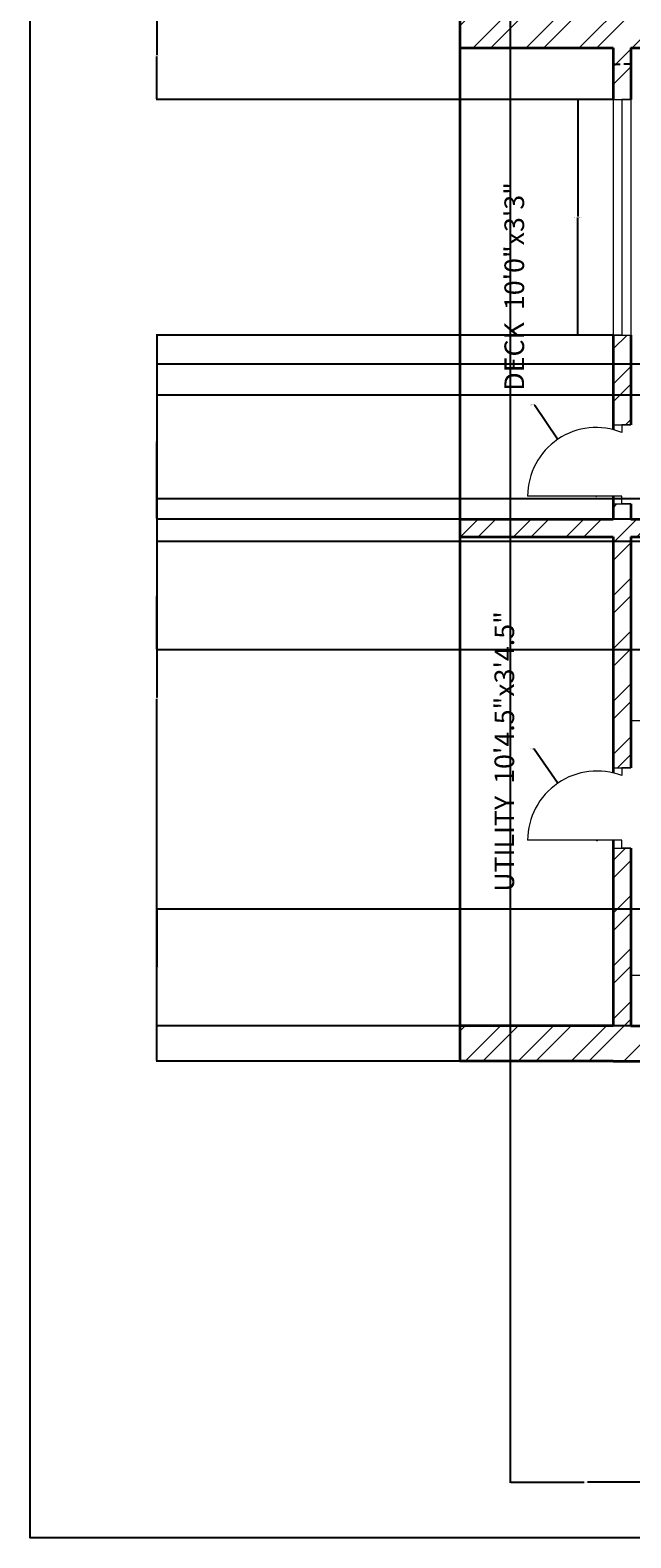
# Model space of a CAD drawing. Units: inches. Extents: x 1748 to 2382, y 1346 to 2284.
# Tile 1 of 26: x 1748 to 1901, y 1346 to 1730. Entities that reach past the tile are written whole.
import ezdxf

# ---------------------------------------------------------------- set-up
doc = ezdxf.new("R2010")
doc.units = ezdxf.units.IN
for name, color, linetype, lineweight in [('A-ANNO-DIMS', 2, 'Continuous', 18), ('A-ANNO-TTLB', 7, 'Continuous', 25), ('A-AREA-IDEN', 7, 'Continuous', 18), ('A-DOOR', 21, 'Continuous', 18), ('A-FLOR-CASE', 32, 'Continuous', 18), ('A-GLAZ', 191, 'Continuous', 18), ('A-WALL', 7, 'Continuous', 35), ('A-WALL-PATT', 9, 'Continuous', 13)]:
    doc.layers.add(name, color=color, linetype=linetype, lineweight=lineweight)
doc.styles.get("Standard").update_dxf_attribs({"font": 'arial.ttf'})
doc.dimstyles.get("Standard").update_dxf_attribs({"dimtxt": 0.18, "dimasz": 0.18, "dimexe": 0.18, "dimexo": 0.0625, "dimgap": 0.09, "dimtad": 0, "dimtih": 1, "dimtoh": 1, "dimdec": 4, "dimzin": 0, "dimdsep": 46, "dimtxsty": 'Standard', "dimcen": 0.09, "dimadec": 0, "dimazin": 0, "dimtfac": 1, "dimtdec": 4, "dimtofl": 0, "dimtmove": 0, "dimatfit": 3, "dimfxl": 1, "dimtolj": 1, "dimtzin": 0, "dimarcsym": 0})

# ---------------------------------------------------------------- blocks, each defined once
blk = doc.blocks.new('WIN-60-SHALLOW')
for p, q in [((0, 60), (4.5, 60)), ((0, 60), (0, 0)), ((4.5, 60), (2.25, 60)), ((2.25, 60), (2.25, 0)), ((4.5, 60), (4.5, 0)), ((2.25, 0), (0, 0)), ((0, 0), (4.5, 0))]:
    blk.add_line(p, q)
blk = doc.blocks.new('*D30')
at = {"layer": 'A-ANNO-DIMS', "color": 0, "lineweight": -2, "transparency": 16777216}
for p, q in [((1896.08, 1712.72), (1886.96, 1712.72)), ((1887.14, 1712.54), (1887.14, 1682.91)), ((1887.14, 1652.9), (1887.14, 1682.54)), ((1896.08, 1652.72), (1886.96, 1652.72))]:
    blk.add_line(p, q, dxfattribs=at)
at = {"layer": 'A-ANNO-DIMS', "color": 0, "transparency": 16777216}
for points in [[(1887.11, 1712.54), (1887.17, 1712.54), (1887.14, 1712.72)], [(1887.11, 1652.9), (1887.17, 1652.9), (1887.14, 1652.72)]]:
    blk.add_solid(points, dxfattribs=at)
at = {"layer": 'Defpoints', "color": 0, "transparency": 16777216}
for p in [(1887.14, 1712.72), (1896.14, 1712.72), (1896.14, 1652.72)]:
    blk.add_point(p, dxfattribs=at)
at = {"layer": 'A-ANNO-DIMS', "color": 0, "transparency": 16777216, "insert": (1887.14, 1682.72), "char_height": 0.18, "attachment_point": 5}
blk.add_mtext('\\A1;WINDOW 60 TYP.', dxfattribs=at)
blk = doc.blocks.new('*D31')
at = {"layer": 'A-ANNO-DIMS', "color": 0, "lineweight": -2, "transparency": 16777216}
for p, q in [((1896.14, 1712.79), (1896.14, 1721.9)), ((1896.32, 1721.72), (1897.93, 1721.72)), ((1900.46, 1721.72), (1898.85, 1721.72)), ((1900.64, 1712.79), (1900.64, 1721.9))]:
    blk.add_line(p, q, dxfattribs=at)
at = {"layer": 'A-ANNO-DIMS', "color": 0, "transparency": 16777216}
for points in [[(1896.32, 1721.75), (1896.32, 1721.69), (1896.14, 1721.72)], [(1900.46, 1721.75), (1900.46, 1721.69), (1900.64, 1721.72)]]:
    blk.add_solid(points, dxfattribs=at)
at = {"layer": 'Defpoints', "color": 0, "transparency": 16777216}
for p in [(1900.64, 1721.72), (1896.14, 1712.72), (1900.64, 1712.72)]:
    blk.add_point(p, dxfattribs=at)
at = {"layer": 'A-ANNO-DIMS', "color": 0, "transparency": 16777216, "insert": (1898.39, 1721.72), "char_height": 0.18, "attachment_point": 5}
blk.add_mtext('\\A1;5 TYP.', dxfattribs=at)
blk = doc.blocks.new('*D42')
at = {"layer": 'A-ANNO-DIMS', "color": 0, "lineweight": -2, "transparency": 16777216}
for p, q in [((1896.08, 1652.72), (1779.88, 1652.72)), ((1780.06, 1652.54), (1780.06, 1560.47)), ((1780.06, 1468.03), (1780.06, 1560.1)), ((1857.08, 1467.85), (1779.88, 1467.85))]:
    blk.add_line(p, q, dxfattribs=at)
at = {"layer": 'A-ANNO-DIMS', "color": 0, "transparency": 16777216}
for points in [[(1780.03, 1652.54), (1780.09, 1652.54), (1780.06, 1652.72)], [(1780.03, 1468.03), (1780.09, 1468.03), (1780.06, 1467.85)]]:
    blk.add_solid(points, dxfattribs=at)
at = {"layer": 'Defpoints', "color": 0, "transparency": 16777216}
for p in [(1780.06, 1652.72), (1896.14, 1652.72), (1857.14, 1467.85)]:
    blk.add_point(p, dxfattribs=at)
at = {"layer": 'A-ANNO-DIMS', "color": 0, "transparency": 16777216, "insert": (1780.06, 1560.29), "char_height": 0.18, "attachment_point": 5}
blk.add_mtext('\\A1;184.87', dxfattribs=at)
blk = doc.blocks.new('*D50')
at = {"layer": 'A-ANNO-DIMS', "color": 0, "lineweight": -2, "transparency": 16777216}
for p, q in [((1869.96, 2223.79), (1869.96, 1360.47)), ((1908.44, 2223.79), (1908.44, 1360.47)), ((1870.14, 1360.65), (1888.81, 1360.65)), ((1908.26, 1360.65), (1889.6, 1360.65))]:
    blk.add_line(p, q, dxfattribs=at)
at = {"layer": 'A-ANNO-DIMS', "color": 0, "transparency": 16777216}
for points in [[(1870.14, 1360.68), (1870.14, 1360.62), (1869.96, 1360.65)], [(1908.26, 1360.68), (1908.26, 1360.62), (1908.44, 1360.65)]]:
    blk.add_solid(points, dxfattribs=at)
at = {"layer": 'Defpoints', "color": 0, "transparency": 16777216}
for p in [(1869.96, 2223.85), (1908.44, 2223.85), (1908.44, 1360.65)]:
    blk.add_point(p, dxfattribs=at)
at = {"layer": 'A-ANNO-DIMS', "color": 0, "transparency": 16777216, "insert": (1889.2, 1360.65), "char_height": 0.18, "attachment_point": 5}
blk.add_mtext('\\A1;38.48', dxfattribs=at)
blk = doc.blocks.new('*D54')
at = {"layer": 'A-ANNO-DIMS', "color": 0, "lineweight": -2, "transparency": 16777216}
for p, q in [((2288.4, 1506.57), (1779.88, 1506.57)), ((1780.06, 1506.39), (1780.06, 1491.89)), ((1780.06, 1477.03), (1780.06, 1491.53)), ((2288.4, 1476.85), (1779.88, 1476.85))]:
    blk.add_line(p, q, dxfattribs=at)
at = {"layer": 'A-ANNO-DIMS', "color": 0, "transparency": 16777216}
for points in [[(1780.03, 1506.39), (1780.09, 1506.39), (1780.06, 1506.57)], [(1780.03, 1477.03), (1780.09, 1477.03), (1780.06, 1476.85)]]:
    blk.add_solid(points, dxfattribs=at)
at = {"layer": 'Defpoints', "color": 0, "transparency": 16777216}
for p in [(1780.06, 1506.57), (2288.46, 1506.57), (2288.46, 1476.85)]:
    blk.add_point(p, dxfattribs=at)
at = {"layer": 'A-ANNO-DIMS', "color": 0, "transparency": 16777216, "insert": (1780.06, 1491.71), "char_height": 0.18, "attachment_point": 5}
blk.add_mtext('\\A1;29.716', dxfattribs=at)
blk = doc.blocks.new('*D55')
at = {"layer": 'A-ANNO-DIMS', "color": 0, "lineweight": -2, "transparency": 16777216}
for p, q in [((2288.4, 1645.3), (1779.88, 1645.3)), ((1780.06, 1645.12), (1780.06, 1625.76)), ((1780.06, 1606.03), (1780.06, 1625.39)), ((2288.4, 1605.85), (1779.88, 1605.85))]:
    blk.add_line(p, q, dxfattribs=at)
at = {"layer": 'A-ANNO-DIMS', "color": 0, "transparency": 16777216}
for points in [[(1780.03, 1645.12), (1780.09, 1645.12), (1780.06, 1645.3)], [(1780.03, 1606.03), (1780.09, 1606.03), (1780.06, 1605.85)]]:
    blk.add_solid(points, dxfattribs=at)
at = {"layer": 'Defpoints', "color": 0, "transparency": 16777216}
for p in [(1780.06, 1645.3), (2288.46, 1645.3), (2288.46, 1605.85)]:
    blk.add_point(p, dxfattribs=at)
at = {"layer": 'A-ANNO-DIMS', "color": 0, "transparency": 16777216, "insert": (1780.06, 1625.58), "char_height": 0.18, "attachment_point": 5}
blk.add_mtext('\\A1;39.454', dxfattribs=at)
blk = doc.blocks.new('*D71')
at = {"layer": 'A-ANNO-DIMS', "color": 0, "lineweight": -2, "transparency": 16777216}
for p, q in [((1857.08, 1734.85), (1779.88, 1734.85)), ((1780.06, 1734.67), (1780.06, 1723.97)), ((1780.06, 1712.9), (1780.06, 1723.61)), ((1896.08, 1712.72), (1779.88, 1712.72))]:
    blk.add_line(p, q, dxfattribs=at)
at = {"layer": 'A-ANNO-DIMS', "color": 0, "transparency": 16777216}
for points in [[(1780.03, 1734.67), (1780.09, 1734.67), (1780.06, 1734.85)], [(1780.03, 1712.9), (1780.09, 1712.9), (1780.06, 1712.72)]]:
    blk.add_solid(points, dxfattribs=at)
at = {"layer": 'Defpoints', "color": 0, "transparency": 16777216}
for p in [(1780.06, 1734.85), (1857.14, 1734.85), (1896.14, 1712.72)]:
    blk.add_point(p, dxfattribs=at)
at = {"layer": 'A-ANNO-DIMS', "color": 0, "transparency": 16777216, "insert": (1780.06, 1723.79), "char_height": 0.18, "attachment_point": 5}
blk.add_mtext('\\A1;22.127', dxfattribs=at)
blk = doc.blocks.new('*D74')
at = {"layer": 'A-ANNO-DIMS', "color": 0, "lineweight": -2, "transparency": 16777216}
for p, q in [((2006.4, 1637.45), (1779.88, 1637.45)), ((1780.06, 1637.27), (1780.06, 1624.43)), ((1780.06, 1611.24), (1780.06, 1624.07)), ((2006.4, 1611.06), (1779.88, 1611.06))]:
    blk.add_line(p, q, dxfattribs=at)
at = {"layer": 'A-ANNO-DIMS', "color": 0, "transparency": 16777216}
for points in [[(1780.03, 1637.27), (1780.09, 1637.27), (1780.06, 1637.45)], [(1780.03, 1611.24), (1780.09, 1611.24), (1780.06, 1611.06)]]:
    blk.add_solid(points, dxfattribs=at)
at = {"layer": 'Defpoints', "color": 0, "transparency": 16777216}
for p in [(1780.06, 1637.45), (2006.46, 1637.45), (2006.46, 1611.06)]:
    blk.add_point(p, dxfattribs=at)
at = {"layer": 'A-ANNO-DIMS', "color": 0, "transparency": 16777216, "insert": (1780.06, 1624.25), "char_height": 0.18, "attachment_point": 5}
blk.add_mtext('\\A1;26.39', dxfattribs=at)
blk = doc.blocks.new('*D80')
at = {"layer": 'A-ANNO-DIMS', "color": 0, "lineweight": -2, "transparency": 16777216}
for p, q in [((2058.9, 1600.19), (1779.88, 1600.19)), ((1780.06, 1600.01), (1780.06, 1586.55)), ((1780.06, 1572.73), (1780.06, 1586.19)), ((2058.9, 1572.55), (1779.88, 1572.55))]:
    blk.add_line(p, q, dxfattribs=at)
at = {"layer": 'A-ANNO-DIMS', "color": 0, "transparency": 16777216}
for points in [[(1780.03, 1600.01), (1780.09, 1600.01), (1780.06, 1600.19)], [(1780.03, 1572.73), (1780.09, 1572.73), (1780.06, 1572.55)]]:
    blk.add_solid(points, dxfattribs=at)
at = {"layer": 'Defpoints', "color": 0, "transparency": 16777216}
for p in [(1780.06, 1600.19), (2058.96, 1600.19), (2058.96, 1572.55)]:
    blk.add_point(p, dxfattribs=at)
at = {"layer": 'A-ANNO-DIMS', "color": 0, "transparency": 16777216, "insert": (1780.06, 1586.37), "char_height": 0.18, "attachment_point": 5}
blk.add_mtext('\\A1;27.637', dxfattribs=at)
blk = doc.blocks.new('*D93')
at = {"layer": 'A-ANNO-DIMS', "color": 0, "lineweight": -2, "transparency": 16777216}
for p, q in [((1875.89, 1547.36), (1876.07, 1547.36)), ((1876.07, 1547.36), (1881.96, 1538.78)), ((1891.95, 1524.08), (1892.13, 1524.08)), ((1892.04, 1523.99), (1892.04, 1524.17))]:
    blk.add_line(p, q, dxfattribs=at)
at = {"layer": 'A-ANNO-DIMS', "color": 0, "transparency": 16777216}
blk.add_solid([(1881.98, 1538.8), (1881.93, 1538.77), (1882.06, 1538.63)], dxfattribs=at)
at = {"layer": 'Defpoints', "color": 0, "transparency": 16777216}
for p in [(1882.06, 1538.63), (1892.04, 1524.08)]:
    blk.add_point(p, dxfattribs=at)
at = {"layer": 'A-ANNO-DIMS', "color": 0, "transparency": 16777216, "insert": (1875.34, 1547.36), "char_height": 0.18, "attachment_point": 5}
blk.add_mtext('\\A1;R17.646', dxfattribs=at)
blk = doc.blocks.new('*D95')
at = {"layer": 'A-ANNO-DIMS', "color": 0, "lineweight": -2, "transparency": 16777216}
for p, q in [((1876.05, 1634.88), (1876.23, 1634.88)), ((1876.23, 1634.88), (1881.99, 1626.34)), ((1891.76, 1611.72), (1891.94, 1611.72)), ((1891.85, 1611.63), (1891.85, 1611.81))]:
    blk.add_line(p, q, dxfattribs=at)
at = {"layer": 'A-ANNO-DIMS', "color": 0, "transparency": 16777216}
blk.add_solid([(1882.01, 1626.36), (1881.96, 1626.32), (1882.09, 1626.19)], dxfattribs=at)
at = {"layer": 'Defpoints', "color": 0, "transparency": 16777216}
for p in [(1882.09, 1626.19), (1891.85, 1611.72)]:
    blk.add_point(p, dxfattribs=at)
at = {"layer": 'A-ANNO-DIMS', "color": 0, "transparency": 16777216, "insert": (1875.5, 1634.88), "char_height": 0.18, "attachment_point": 5}
blk.add_mtext('\\A1;R17.458', dxfattribs=at)

msp = doc.modelspace()

# ---------------------------------------------------------------- hatches: boundary and pattern name
at = {"layer": 'A-WALL-PATT'}
h = msp.add_hatch(dxfattribs=at)
h.set_pattern_fill('ANSI32', color=256)
h.paths.add_polyline_path([(1908.4445, 2232.8497), (1821.9607, 2232.8497), (1821.9607, 2223.8497), (1865.4607, 2223.8497), (1865.4607, 2209.9185), (1869.9607, 2209.9185), (1869.9607, 2223.8497), (1908.4445, 2223.8497), (1908.4445, 2228.3497)])
h.paths.add_polyline_path([(2040.0683, 2232.8497), (1968.4445, 2232.8497), (1968.4445, 2223.8497), (2025.9607, 2223.8497), (2025.9607, 2130.3497), (2032.1341, 2130.3497), (2032.1341, 2132.5997), (2032.1341, 2134.8497), (2030.4607, 2134.8497), (2030.4607, 2223.8497), (2040.0683, 2223.8497)])
h.paths.add_polyline_path([(2091.3969, 2232.8497), (2064.0683, 2232.8497), (2064.0683, 2223.8497), (2078.4607, 2223.8497), (2078.4607, 2134.8497), (2051.1563, 2134.8497), (2051.1563, 2130.3497), (2078.4607, 2130.3497), (2078.4607, 2128.6813), (2082.9607, 2128.6813), (2082.9607, 2130.3497), (2086.1879, 2130.3497), (2086.1879, 2132.5997), (2086.1879, 2134.8497), (2082.9607, 2134.8497), (2082.9607, 2223.8497), (2091.3969, 2223.8497), (2091.3969, 2228.3497)])
h.paths.add_polyline_path([(2167.0164, 2232.8497), (2115.3969, 2232.8497), (2115.3969, 2223.8497), (2130.9607, 2223.8497), (2130.9607, 2134.8497), (2106.9607, 2134.8497), (2106.9607, 2130.3497), (2135.4607, 2130.3497), (2135.4607, 2223.8497), (2167.0164, 2223.8497), (2167.0164, 2228.3497)])
h.paths.add_polyline_path([(1869.9607, 2149.9185), (1865.4607, 2149.9185), (1865.4607, 2127.8942), (1869.9607, 2127.8942)])
h.paths.add_polyline_path([(2082.9607, 2104.4871), (2080.7107, 2104.4871), (2078.4607, 2104.4871), (2078.4607, 2103.8497), (1869.9607, 2103.8497), (1869.9607, 2108.6062), (1867.7107, 2108.6062), (1865.4607, 2108.6062), (1865.4607, 2103.8497), (1821.9607, 2103.8497), (1821.9607, 2099.3497), (1865.4607, 2099.3497), (1865.4607, 2094.7509), (1869.9607, 2094.7509), (1869.9607, 2099.3497), (2025.9607, 2099.3497), (2025.9607, 2096.4326), (2030.4607, 2096.4326), (2030.4607, 2099.3497), (2082.9607, 2099.3497)])
h.paths.add_polyline_path([(1928.9457, 1401.1212), (2176.8693, 1401.1212), (2176.8693, 1438.214), (1928.9457, 1438.214)], flags=9)
h.paths.add_polyline_path([(2122.2668, 2048.1927), (2177.9387, 2048.1927), (2177.9387, 2066.85), (2122.2668, 2066.85)], flags=9)
h.paths.add_polyline_path([(2272.688, 2153.8197), (2272.688, 2216.746), (2262.3845, 2216.746), (2262.3845, 2153.8197)], flags=9)
h.paths.add_polyline_path([(2157.2928, 2166.5593), (2196.3822, 2166.5593), (2196.3822, 2185.2167), (2157.2928, 2185.2167)], flags=9)
h.paths.add_polyline_path([(2089.3407, 2162.0698), (2124.3987, 2162.0698), (2124.3987, 2180.7272), (2089.3407, 2180.7272)], flags=9)
h.paths.add_polyline_path([(2037.4521, 2160.0913), (2072.5101, 2160.0913), (2072.5101, 2178.7486), (2037.4521, 2178.7486)], flags=9)
h.paths.add_polyline_path([(1884.7894, 2104.1554), (1923.6297, 2104.1554), (1923.6297, 2122.8127), (1884.7894, 2122.8127)], flags=9)
h.paths.add_polyline_path([(1851.2832, 2142.9749), (1851.2832, 2199.3051), (1840.9796, 2199.3051), (1840.9796, 2142.9749)], flags=9)
h.paths.add_polyline_path([(1844.8763, 2017.2834), (1844.8763, 2073.6136), (1834.5728, 2073.6136), (1834.5728, 2017.2834)], flags=9)
h.paths.add_polyline_path([(1897.1577, 2073.1279), (1935.9981, 2073.1279), (1935.9981, 2091.7853), (1897.1577, 2091.7853)], flags=9)
h.paths.add_polyline_path([(1952.3395, 1802.4231), (2008.0114, 1802.4231), (2008.0114, 1821.0805), (1952.3395, 1821.0805)], flags=9)
h.paths.add_polyline_path([(1978.8184, 1857.6841), (2017.7338, 1857.6841), (2017.7338, 1876.3415), (1978.8184, 1876.3415)], flags=9)
h.paths.add_polyline_path([(1979.6513, 1925.9516), (2008.8089, 1925.9516), (2008.8089, 1944.6089), (1979.6513, 1944.6089)], flags=9)
h.paths.add_polyline_path([(1838.5553, 1860.3527), (1877.3957, 1860.3527), (1877.3957, 1879.01), (1838.5553, 1879.01)], flags=9)
h.paths.add_polyline_path([(1883.9018, 1787.3013), (1883.9018, 1843.6315), (1873.5983, 1843.6315), (1873.5983, 1787.3013)], flags=9)
h.paths.add_polyline_path([(1873.7079, 1509.1938), (1873.7079, 1583.7709), (1863.4044, 1583.7709), (1863.4044, 1509.1938)], flags=9)
h.paths.add_polyline_path([(1916.2259, 1603.3681), (1955.0663, 1603.3681), (1955.0663, 1622.0254), (1916.2259, 1622.0254)], flags=9)
h.paths.add_polyline_path([(1876.3013, 1636.757), (1876.3013, 1693.0871), (1865.9978, 1693.0871), (1865.9978, 1636.757)], flags=9)
h.paths.add_polyline_path([(1921.3138, 1521.8316), (1964.0662, 1521.8316), (1964.0662, 1540.489), (1921.3138, 1540.489)], flags=9)
h.paths.add_polyline_path([(2017.5657, 1497.5078), (2046.7983, 1497.5078), (2046.7983, 1516.1651), (2017.5657, 1516.1651)], flags=9)
h.paths.add_polyline_path([(2066.8661, 1499.3902), (2096.0988, 1499.3902), (2096.0988, 1518.0475), (2066.8661, 1518.0475)], flags=9)
h.paths.add_polyline_path([(2155.4835, 1571.6596), (2198.2358, 1571.6596), (2198.2358, 1590.3169), (2155.4835, 1590.3169)], flags=9)
h.paths.add_polyline_path([(2094.9136, 1664.6812), (2150.5855, 1664.6812), (2150.5855, 1683.3386), (2094.9136, 1683.3386)], flags=9)
h.paths.add_polyline_path([(2257.6902, 1863.1628), (2269.8935, 1863.1628), (2269.8935, 1873.4664), (2257.6902, 1873.4664)], flags=9)
h.paths.add_polyline_path([(2164.0748, 1880.3089), (2189.8694, 1880.3089), (2189.8694, 1890.6124), (2164.0748, 1890.6124)], flags=9)
h.paths.add_polyline_path([(2239.4394, 1931.0585), (2268.8187, 1931.0585), (2268.8187, 1949.7159), (2239.4394, 1949.7159)], flags=9)
h = msp.add_hatch(dxfattribs=at)
h.set_pattern_fill('ANSI32', color=256)
h.paths.add_polyline_path([(2297.4607, 2232.8497), (2203.0164, 2232.8497), (2203.0164, 2223.8497), (2244.9607, 2223.8497), (2244.9607, 2127.8554), (2249.4607, 2127.8554), (2249.4607, 2223.8497), (2297.4607, 2223.8497)])
h.paths.add_polyline_path([(2297.4607, 2103.8497), (2249.4607, 2103.8497), (2249.4607, 2106.7497), (2247.2107, 2106.7497), (2244.9607, 2106.7497), (2244.9607, 2103.8497), (2130.9607, 2103.8497), (2130.9607, 2099.3497), (2288.4607, 2099.3497), (2288.4607, 2077.2008), (2297.4607, 2077.2008)])
h.paths.add_polyline_path([(1928.9457, 1401.1212), (2176.8693, 1401.1212), (2176.8693, 1438.214), (1928.9457, 1438.214)], flags=9)
h.paths.add_polyline_path([(2122.2668, 2048.1927), (2177.9387, 2048.1927), (2177.9387, 2066.85), (2122.2668, 2066.85)], flags=9)
h.paths.add_polyline_path([(2272.688, 2153.8197), (2272.688, 2216.746), (2262.3845, 2216.746), (2262.3845, 2153.8197)], flags=25)
h.paths.add_polyline_path([(2157.2928, 2166.5593), (2196.3822, 2166.5593), (2196.3822, 2185.2167), (2157.2928, 2185.2167)], flags=9)
h.paths.add_polyline_path([(2089.3407, 2162.0698), (2124.3987, 2162.0698), (2124.3987, 2180.7272), (2089.3407, 2180.7272)], flags=9)
h.paths.add_polyline_path([(2037.4521, 2160.0913), (2072.5101, 2160.0913), (2072.5101, 2178.7486), (2037.4521, 2178.7486)], flags=9)
h.paths.add_polyline_path([(1884.7894, 2104.1554), (1923.6297, 2104.1554), (1923.6297, 2122.8127), (1884.7894, 2122.8127)], flags=9)
h.paths.add_polyline_path([(1851.2832, 2142.9749), (1851.2832, 2199.3051), (1840.9796, 2199.3051), (1840.9796, 2142.9749)], flags=9)
h.paths.add_polyline_path([(1844.8763, 2017.2834), (1844.8763, 2073.6136), (1834.5728, 2073.6136), (1834.5728, 2017.2834)], flags=9)
h.paths.add_polyline_path([(1897.1577, 2073.1279), (1935.9981, 2073.1279), (1935.9981, 2091.7853), (1897.1577, 2091.7853)], flags=9)
h.paths.add_polyline_path([(1952.3395, 1802.4231), (2008.0114, 1802.4231), (2008.0114, 1821.0805), (1952.3395, 1821.0805)], flags=9)
h.paths.add_polyline_path([(1978.8184, 1857.6841), (2017.7338, 1857.6841), (2017.7338, 1876.3415), (1978.8184, 1876.3415)], flags=9)
h.paths.add_polyline_path([(1979.6513, 1925.9516), (2008.8089, 1925.9516), (2008.8089, 1944.6089), (1979.6513, 1944.6089)], flags=9)
h.paths.add_polyline_path([(1838.5553, 1860.3527), (1877.3957, 1860.3527), (1877.3957, 1879.01), (1838.5553, 1879.01)], flags=9)
h.paths.add_polyline_path([(1883.9018, 1787.3013), (1883.9018, 1843.6315), (1873.5983, 1843.6315), (1873.5983, 1787.3013)], flags=9)
h.paths.add_polyline_path([(1873.7079, 1509.1938), (1873.7079, 1583.7709), (1863.4044, 1583.7709), (1863.4044, 1509.1938)], flags=9)
h.paths.add_polyline_path([(1916.2259, 1603.3681), (1955.0663, 1603.3681), (1955.0663, 1622.0254), (1916.2259, 1622.0254)], flags=9)
h.paths.add_polyline_path([(1876.3013, 1636.757), (1876.3013, 1693.0871), (1865.9978, 1693.0871), (1865.9978, 1636.757)], flags=9)
h.paths.add_polyline_path([(1921.3138, 1521.8316), (1964.0662, 1521.8316), (1964.0662, 1540.489), (1921.3138, 1540.489)], flags=9)
h.paths.add_polyline_path([(2017.5657, 1497.5078), (2046.7983, 1497.5078), (2046.7983, 1516.1651), (2017.5657, 1516.1651)], flags=9)
h.paths.add_polyline_path([(2066.8661, 1499.3902), (2096.0988, 1499.3902), (2096.0988, 1518.0475), (2066.8661, 1518.0475)], flags=9)
h.paths.add_polyline_path([(2155.4835, 1571.6596), (2198.2358, 1571.6596), (2198.2358, 1590.3169), (2155.4835, 1590.3169)], flags=9)
h.paths.add_polyline_path([(2094.9136, 1664.6812), (2150.5855, 1664.6812), (2150.5855, 1683.3386), (2094.9136, 1683.3386)], flags=9)
h.paths.add_polyline_path([(2257.6902, 1863.1628), (2269.8935, 1863.1628), (2269.8935, 1873.4664), (2257.6902, 1873.4664)], flags=9)
h.paths.add_polyline_path([(2164.0748, 1880.3089), (2189.8694, 1880.3089), (2189.8694, 1890.6124), (2164.0748, 1890.6124)], flags=9)
h.paths.add_polyline_path([(2239.4394, 1931.0585), (2268.8187, 1931.0585), (2268.8187, 1949.7159), (2239.4394, 1949.7159)], flags=9)
h = msp.add_hatch(dxfattribs=at)
h.set_pattern_fill('ANSI32', color=256)
h.paths.add_polyline_path([(1919.6777, 1476.8497), (1900.6426, 1476.8497), (1900.6426, 1522.0826), (1898.3926, 1522.0826), (1896.1426, 1522.0826), (1896.1426, 1476.8497), (1857.1426, 1476.8497), (1857.1426, 1467.8497), (1896.1426, 1467.8497), (1919.6777, 1467.8497), (1919.6777, 1472.3497)])
h.paths.add_polyline_path([(2018.7873, 1472.3497), (2018.7873, 1476.8497), (2010.9607, 1476.8497), (2010.9607, 1560.8497), (2034.9607, 1560.8497), (2034.9607, 1565.3497), (2006.4607, 1565.3497), (2006.4607, 1476.8497), (1955.6777, 1476.8497), (1955.6777, 1467.8497), (2018.7873, 1467.8497)])
h.paths.add_polyline_path([(2152.3354, 1472.3497), (2152.3354, 1476.8497), (2115.9607, 1476.8497), (2115.9607, 1565.3497), (2109.2204, 1565.3497), (2109.2204, 1563.0997), (2109.2204, 1560.8497), (2111.4607, 1560.8497), (2111.4607, 1476.8497), (2095.3617, 1476.8497), (2095.3617, 1467.8497), (2152.3354, 1467.8497)])
h.paths.add_polyline_path([(2071.3617, 1476.8497), (2063.4607, 1476.8497), (2063.4607, 1560.8497), (2090.1865, 1560.8497), (2090.1865, 1565.3497), (2063.4607, 1565.3497), (2063.4607, 1572.5485), (2061.2107, 1572.5485), (2058.9607, 1572.5485), (2058.9607, 1565.3497), (2055.6281, 1565.3497), (2055.6281, 1560.8497), (2058.9607, 1560.8497), (2058.9607, 1476.8497), (2042.7873, 1476.8497), (2042.7873, 1467.8497), (2071.3617, 1467.8497), (2071.3617, 1472.3497)])
h.paths.add_polyline_path([(2297.4607, 1506.5652), (2288.4607, 1506.5652), (2288.4607, 1476.8497), (2212.3354, 1476.8497), (2212.3354, 1467.8497), (2297.4607, 1467.8497)])
h.paths.add_polyline_path([(2297.4607, 1645.3038), (2288.4607, 1645.3038), (2288.4607, 1605.8497), (2058.9607, 1605.8497), (2058.9607, 1600.1857), (2061.2107, 1600.1857), (2063.4607, 1600.1857), (2063.4607, 1601.3497), (2288.4607, 1601.3497), (2288.4607, 1566.5652), (2297.4607, 1566.5652)])
h.paths.add_polyline_path([(2010.9607, 1609.0561), (2008.7107, 1609.0561), (2006.4607, 1609.0561), (2006.4607, 1605.8497), (1900.6426, 1605.8497), (1900.6426, 1609.7171), (1898.3926, 1609.7171), (1896.1426, 1609.7171), (1896.1426, 1605.8497), (1857.1426, 1605.8497), (1857.1426, 1601.3497), (1896.1426, 1601.3497), (1896.1426, 1542.5447), (1900.6426, 1542.5447), (1900.6426, 1601.3497), (2010.9607, 1601.3497)])
h.paths.add_polyline_path([(1928.9457, 1401.1212), (2176.8693, 1401.1212), (2176.8693, 1438.214), (1928.9457, 1438.214)], flags=9)
h.paths.add_polyline_path([(2122.2668, 2048.1927), (2177.9387, 2048.1927), (2177.9387, 2066.85), (2122.2668, 2066.85)], flags=9)
h.paths.add_polyline_path([(2272.688, 2153.8197), (2272.688, 2216.746), (2262.3845, 2216.746), (2262.3845, 2153.8197)], flags=9)
h.paths.add_polyline_path([(2157.2928, 2166.5593), (2196.3822, 2166.5593), (2196.3822, 2185.2167), (2157.2928, 2185.2167)], flags=9)
h.paths.add_polyline_path([(2089.3407, 2162.0698), (2124.3987, 2162.0698), (2124.3987, 2180.7272), (2089.3407, 2180.7272)], flags=9)
h.paths.add_polyline_path([(2037.4521, 2160.0913), (2072.5101, 2160.0913), (2072.5101, 2178.7486), (2037.4521, 2178.7486)], flags=9)
h.paths.add_polyline_path([(1884.7894, 2104.1554), (1923.6297, 2104.1554), (1923.6297, 2122.8127), (1884.7894, 2122.8127)], flags=9)
h.paths.add_polyline_path([(1851.2832, 2142.9749), (1851.2832, 2199.3051), (1840.9796, 2199.3051), (1840.9796, 2142.9749)], flags=9)
h.paths.add_polyline_path([(1844.8763, 2017.2834), (1844.8763, 2073.6136), (1834.5728, 2073.6136), (1834.5728, 2017.2834)], flags=9)
h.paths.add_polyline_path([(1897.1577, 2073.1279), (1935.9981, 2073.1279), (1935.9981, 2091.7853), (1897.1577, 2091.7853)], flags=9)
h.paths.add_polyline_path([(1952.3395, 1802.4231), (2008.0114, 1802.4231), (2008.0114, 1821.0805), (1952.3395, 1821.0805)], flags=9)
h.paths.add_polyline_path([(1978.8184, 1857.6841), (2017.7338, 1857.6841), (2017.7338, 1876.3415), (1978.8184, 1876.3415)], flags=9)
h.paths.add_polyline_path([(1979.6513, 1925.9516), (2008.8089, 1925.9516), (2008.8089, 1944.6089), (1979.6513, 1944.6089)], flags=9)
h.paths.add_polyline_path([(1838.5553, 1860.3527), (1877.3957, 1860.3527), (1877.3957, 1879.01), (1838.5553, 1879.01)], flags=9)
h.paths.add_polyline_path([(1883.9018, 1787.3013), (1883.9018, 1843.6315), (1873.5983, 1843.6315), (1873.5983, 1787.3013)], flags=9)
h.paths.add_polyline_path([(1873.7079, 1509.1938), (1873.7079, 1583.7709), (1863.4044, 1583.7709), (1863.4044, 1509.1938)], flags=9)
h.paths.add_polyline_path([(1916.2259, 1603.3681), (1955.0663, 1603.3681), (1955.0663, 1622.0254), (1916.2259, 1622.0254)], flags=9)
h.paths.add_polyline_path([(1876.3013, 1636.757), (1876.3013, 1693.0871), (1865.9978, 1693.0871), (1865.9978, 1636.757)], flags=9)
h.paths.add_polyline_path([(1921.3138, 1521.8316), (1964.0662, 1521.8316), (1964.0662, 1540.489), (1921.3138, 1540.489)], flags=9)
h.paths.add_polyline_path([(2017.5657, 1497.5078), (2046.7983, 1497.5078), (2046.7983, 1516.1651), (2017.5657, 1516.1651)], flags=9)
h.paths.add_polyline_path([(2066.8661, 1499.3902), (2096.0988, 1499.3902), (2096.0988, 1518.0475), (2066.8661, 1518.0475)], flags=9)
h.paths.add_polyline_path([(2155.4835, 1571.6596), (2198.2358, 1571.6596), (2198.2358, 1590.3169), (2155.4835, 1590.3169)], flags=25)
h.paths.add_polyline_path([(2094.9136, 1664.6812), (2150.5855, 1664.6812), (2150.5855, 1683.3386), (2094.9136, 1683.3386)], flags=9)
h.paths.add_polyline_path([(2257.6902, 1863.1628), (2269.8935, 1863.1628), (2269.8935, 1873.4664), (2257.6902, 1873.4664)], flags=9)
h.paths.add_polyline_path([(2164.0748, 1880.3089), (2189.8694, 1880.3089), (2189.8694, 1890.6124), (2164.0748, 1890.6124)], flags=9)
h.paths.add_polyline_path([(2239.4394, 1931.0585), (2268.8187, 1931.0585), (2268.8187, 1949.7159), (2239.4394, 1949.7159)], flags=9)
h = msp.add_hatch(dxfattribs=at)
h.set_pattern_fill('ANSI32', color=256)
h.paths.add_polyline_path([(1900.6426, 1652.723), (1896.1426, 1652.723), (1896.1426, 1629.9029), (1900.6426, 1629.9029)])
h.paths.add_polyline_path([(2206.0699, 1859.3497), (2197.0699, 1859.3497), (2197.0699, 1734.8497), (2206.0699, 1734.8497)], flags=17)
h.paths.add_polyline_path([(2297.4607, 1865.3269), (2288.4607, 1865.3269), (2288.4607, 1734.8497), (2206.0699, 1734.8497), (2180.4551, 1734.8497), (2180.4551, 1725.8497), (2197.0699, 1725.8497), (2206.0699, 1725.8497), (2288.4607, 1725.8497), (2288.4607, 1705.3038), (2297.4607, 1705.3038)])
h.paths.add_polyline_path([(2139.9607, 1815.8001), (2135.4607, 1815.8001), (2130.9607, 1815.8001), (2130.9607, 1734.8497), (1900.6426, 1734.8497), (1900.6426, 1738.9477), (1898.3926, 1738.9477), (1896.1426, 1738.9477), (1896.1426, 1734.8497), (1857.1426, 1734.8497), (1857.1426, 1725.8497), (1896.1426, 1725.8497), (1896.1426, 1712.723), (1900.6426, 1712.723), (1900.6426, 1725.8497), (2006.4607, 1725.8497), (2006.4607, 1637.448), (2010.9607, 1637.448), (2010.9607, 1725.8497), (2139.9607, 1725.8497), (2147.389, 1725.8497), (2147.389, 1730.3497), (2147.389, 1734.8497), (2139.9607, 1734.8497)])
h.paths.add_polyline_path([(2149.8497, 1917.8497), (2149.8497, 1922.3497), (2139.9607, 1922.3497), (2139.9607, 1979.3497), (2030.4607, 1979.3497), (2030.4607, 2069.8971), (2028.2107, 2069.8971), (2025.9607, 2069.8971), (2025.9607, 1979.3497), (1869.9607, 1979.3497), (1869.9607, 1998.93), (1865.4607, 1998.93), (1865.4607, 1979.3497), (1821.9607, 1979.3497), (1821.9607, 1952.7922), (1826.9306, 1952.7922), (1830.9607, 1952.7922), (1830.9607, 1970.3497), (1962.9607, 1970.3497), (1962.9607, 1926.5713), (1967.4607, 1926.5713), (1967.4607, 1970.3497), (2027.4607, 1970.3497), (2027.4607, 1898.3497), (2004.9604, 1898.3497), (2004.9604, 1893.8497), (2027.4607, 1893.8497), (2027.4607, 1859.3497), (1958.8973, 1859.3497), (1958.8973, 1854.8497), (2047.917, 1854.8497), (2047.917, 1859.3497), (2031.9607, 1859.3497), (2031.9607, 1970.3497), (2130.9607, 1970.3497), (2130.9607, 1859.3497), (2104.9565, 1859.3497), (2104.9565, 1854.8497), (2130.9607, 1854.8497), (2130.9607, 1849.0684), (2139.9607, 1849.0684), (2139.9607, 1913.3497), (2149.8497, 1913.3497)])
h.paths.add_polyline_path([(1928.9996, 1859.3497), (1830.9607, 1859.3497), (1830.9607, 1892.7922), (1821.9607, 1892.7922), (1821.9607, 1854.8497), (1896.1426, 1854.8497), (1896.1426, 1836.6443), (1898.378, 1836.6443), (1900.6426, 1836.6443), (1900.6426, 1854.8497), (1928.9996, 1854.8497), (1928.9996, 1857.0997)])
h.paths.add_polyline_path([(1980.9604, 1896.0997), (1980.9604, 1898.3497), (1967.4607, 1898.3497), (1967.4607, 1902.3846), (1962.9607, 1902.3846), (1962.9607, 1859.3497), (1967.4607, 1859.3497), (1967.4607, 1893.8497), (1980.9604, 1893.8497)], flags=17)
h.paths.add_polyline_path([(1900.6426, 1776.6443), (1896.1426, 1776.6443), (1896.1426, 1758.0891), (1900.6426, 1758.0891)], flags=17)
h.paths.add_polyline_path([(2297.4607, 2017.2008), (2288.4607, 2017.2008), (2288.4607, 1979.3497), (2213.4607, 1979.3497), (2213.4607, 1922.3497), (2183.3516, 1922.3497), (2183.3516, 1913.3497), (2213.4607, 1913.3497), (2236.234, 1913.3497), (2236.234, 1922.3497), (2222.4607, 1922.3497), (2222.4607, 1931.3497), (2222.4607, 1970.3497), (2288.4607, 1970.3497), (2288.4607, 1922.3497), (2272.1921, 1922.3497), (2272.1921, 1913.3497), (2288.4607, 1913.3497), (2288.4607, 1901.3269), (2297.4607, 1901.3269)])

# ---------------------------------------------------------------- linework, layer by layer
at = {"layer": 'A-ANNO-TTLB'}
msp.add_lwpolyline([(1747.8112, 2284.3704), (2382.1361, 2284.3704), (2382.1361, 1346.4899), (1747.8112, 1346.4899)], close=True, dxfattribs=at)
at = {"layer": 'A-DOOR'}
for p, q in [((1896.1426, 1629.9029), (1900.6426, 1629.9029)), ((1900.6426, 1629.9029), (1898.3926, 1629.9029)), ((1898.3926, 1629.9029), (1898.3926, 1627.9029)), ((1898.3926, 1611.7171), (1874.3926, 1611.7171)), ((1896.1426, 1609.7171), (1900.6426, 1609.7171)), ((1898.3926, 1609.7171), (1898.3926, 1611.7171)), ((1900.6426, 1609.7171), (1898.3926, 1609.7171)), ((1896.1426, 1542.5447), (1900.6426, 1542.5447)), ((1900.6426, 1542.5447), (1898.3926, 1542.5447)), ((1898.3926, 1542.5447), (1898.3926, 1540.5447)), ((1898.3926, 1524.0826), (1874.3926, 1524.0826)), ((1898.3926, 1522.0826), (1898.3926, 1524.0826)), ((1896.1426, 1522.0826), (1900.6426, 1522.0826)), ((1900.6426, 1522.0826), (1898.3926, 1522.0826))]:
    msp.add_line(p, q, dxfattribs=at)
for centre, radius, start in [((1891.8506, 1611.7171), 17.4579, 67.992126), ((1892.0385, 1524.0826), 17.6458, 68.893972)]:
    msp.add_arc(centre, radius, start, 180, dxfattribs=at)
at = {"layer": 'A-FLOR-CASE'}
for p, q in [((1900.6426, 1554.5909), (1908.5437, 1554.5909)), ((1900.6426, 1489.7224), (2006.4607, 1489.7224))]:
    msp.add_line(p, q, dxfattribs=at)
at = {"layer": 'A-WALL'}
for p, q in [((1857.1426, 1854.8497), (1857.1426, 1605.8497)), ((1857.1426, 1725.8497), (1896.1426, 1725.8497)), ((1896.1426, 1725.8497), (1896.1426, 1712.723)), ((1900.6426, 1725.8497), (1900.6426, 1712.723)), ((1900.6426, 1725.8497), (2006.4607, 1725.8497)), ((1896.1426, 1652.723), (1896.1426, 1628.6392)), ((1900.6426, 1652.723), (1900.6426, 1629.9029)), ((1896.1426, 1611.7171), (1896.1426, 1605.8497)), ((1900.6426, 1609.7171), (1900.6426, 1605.8497)), ((1857.1426, 1605.8497), (1896.1426, 1605.8497)), ((1857.1426, 1605.8497), (1857.1426, 1467.8497)), ((1900.6426, 1605.8497), (2006.4607, 1605.8497)), ((1857.1426, 1601.3497), (1896.1426, 1601.3497)), ((1896.1426, 1601.3497), (1896.1426, 1541.2445)), ((1900.6426, 1601.3497), (1900.6426, 1542.5447)), ((1900.6426, 1601.3497), (2010.9607, 1601.3497)), ((1896.1426, 1524.0826), (1896.1426, 1476.8497)), ((1900.6426, 1522.0826), (1900.6426, 1476.8497)), ((1896.1426, 1476.8497), (1857.1426, 1476.8497)), ((1900.6426, 1476.8497), (1919.6777, 1476.8497)), ((1896.1426, 1467.8497), (1857.1426, 1467.8497)), ((1896.1426, 1467.8497), (1919.6777, 1467.8497))]:
    msp.add_line(p, q, dxfattribs=at)

# ---------------------------------------------------------------- block references
at = {"layer": 'A-GLAZ'}
msp.add_blockref('WIN-60-SHALLOW', (1896.143, 1652.723), dxfattribs=at)

# ---------------------------------------------------------------- texts
at = {"layer": 'A-AREA-IDEN', "char_height": 5, "attachment_point": 1, "rotation": 90}
for s, width, insert in [('DECK  10\'0"x3\'3"', 159.777871, (1868.4859, 1638.5458)), ('UTILITY  10\'4.5"x3\'4.5"', 394.394912, (1865.9572, 1510.993))]:
    msp.add_mtext_dynamic_manual_height_columns(s, width=width, gutter_width=12.5, heights=[0], dxfattribs=dict(at, insert=insert))

# ---------------------------------------------------------------- dimensions: what is measured, and where the dimension line sits
at = {"layer": 'A-ANNO-DIMS'}
dim = msp.add_linear_dim(base=(1908.4445, 1360.6451), p1=(1869.9607, 2223.8497), p2=(1908.4445, 2223.8497), dimstyle='Standard', override={"dimdec": 2, "dimlfac": 1, "dimrnd": 0, "dimzin": 0, "dimdsep": 46, "dimlunit": 2}, dxfattribs=at)
dim.commit()
dim.dimension.update_dxf_attribs({"geometry": '*D50', "text_midpoint": (1889.2026, 1360.6451)})
for base, p1, p2, override, picture, middle in [((1780.0607, 1734.8497), (1896.1426, 1712.723), (1857.1426, 1734.8497), {"dimdec": 3, "dimlfac": 1, "dimrnd": 0, "dimzin": 0, "dimdsep": 46, "dimlunit": 2}, '*D71', (1780.0607, 1723.7863)), ((1780.0607, 1652.723), (1857.1426, 1467.8497), (1896.1426, 1652.723), {"dimdec": 2, "dimlfac": 1, "dimrnd": 0, "dimzin": 0, "dimdsep": 46, "dimlunit": 2}, '*D42', (1780.0607, 1560.2863)), ((1780.0607, 1645.3038), (2288.4607, 1605.8497), (2288.4607, 1645.3038), {"dimdec": 3, "dimlfac": 1, "dimrnd": 0, "dimzin": 0, "dimdsep": 46, "dimlunit": 2}, '*D55', (1780.0607, 1625.5767)), ((1780.0607, 1637.448), (2006.4607, 1611.0561), (2006.4607, 1637.448), {"dimdec": 2, "dimlfac": 1, "dimrnd": 0, "dimzin": 0, "dimdsep": 46, "dimlunit": 2}, '*D74', (1780.0607, 1624.252)), ((1780.0607, 1600.1857), (2058.9607, 1572.5485), (2058.9607, 1600.1857), {"dimdec": 3, "dimlfac": 1, "dimrnd": 0, "dimzin": 0, "dimdsep": 46, "dimlunit": 2}, '*D80', (1780.0607, 1586.3671)), ((1780.06066, 1506.56516), (2288.46066, 1476.84965), (2288.46066, 1506.56516), {"dimdec": 3, "dimlfac": 1, "dimrnd": 0, "dimzin": 0, "dimdsep": 46, "dimlunit": 2}, '*D54', (1780.06066, 1491.7074))]:
    dim = msp.add_linear_dim(base=base, p1=p1, p2=p2, angle=90, dimstyle='Standard', override=override, dxfattribs=at)
    dim.commit()
    dim.dimension.update_dxf_attribs({"geometry": picture, "text_midpoint": middle})
dim = msp.add_linear_dim(base=(1900.642649623, 1721.7230454755), p1=(1896.142649623, 1712.7230454755), p2=(1900.642649623, 1712.7230454755), text='<> TYP.', dimstyle='Standard', override={"dimdec": 0, "dimlfac": 1, "dimrnd": 0, "dimzin": 0, "dimdsep": 46, "dimlunit": 2}, dxfattribs=at)
dim.commit()
dim.dimension.update_dxf_attribs({"geometry": '*D31', "text_midpoint": (1898.392649623, 1721.7230454755)})
dim = msp.add_linear_dim(base=(1887.1426, 1712.723), p1=(1896.1426, 1652.723), p2=(1896.1426, 1712.723), angle=90, text='WINDOW <> TYP.', dimstyle='Standard', override={"dimdec": 0, "dimlfac": 1, "dimrnd": 0, "dimzin": 0, "dimdsep": 46, "dimlunit": 2}, dxfattribs=at)
dim.commit()
dim.dimension.update_dxf_attribs({"geometry": '*D30', "text_midpoint": (1887.1426, 1682.723)})
for center, mpoint, picture, middle in [((1891.8506, 1611.7171), (1882.089, 1626.191), '*D95', (1875.5022, 1634.8752)), ((1892.0385, 1524.0826), (1882.0569, 1538.6341), '*D93', (1875.3383, 1547.3649))]:
    dim = msp.add_radius_dim(center=center, mpoint=mpoint, dimstyle='Standard', override={"dimdec": 3, "dimlfac": 1, "dimrnd": 0, "dimzin": 0, "dimdsep": 46, "dimlunit": 2}, dxfattribs=at)
    dim.commit()
    dim.dimension.update_dxf_attribs({"geometry": picture, "text_midpoint": middle, "dimtype": 164})

doc.saveas('drawing.dxf')
